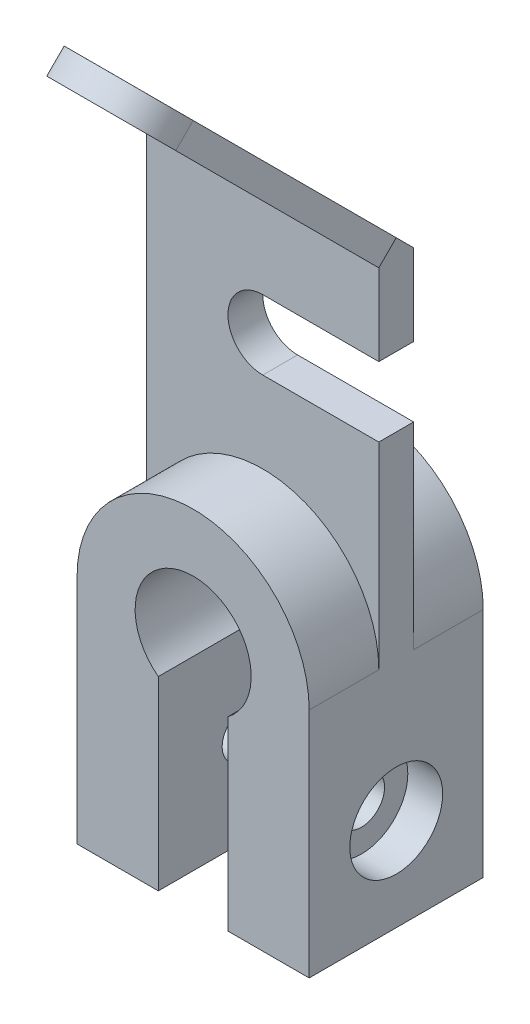
ISO-10303-21;
HEADER;
FILE_DESCRIPTION(('STEP AP214'),'2;1');
FILE_NAME('part.step','',(''),(''),'','','');
FILE_SCHEMA(('AUTOMOTIVE_DESIGN { 1 0 10303 214 1 1 1 1 }'));
ENDSEC;
DATA;
#1=APPLICATION_CONTEXT('core data for automotive mechanical design processes');
#2=APPLICATION_PROTOCOL_DEFINITION('international standard','automotive_design',2000,#1);
#3=PRODUCT_CONTEXT('',#1,'mechanical');
#4=PRODUCT('Part','Part','',(#3));
#5=PRODUCT_RELATED_PRODUCT_CATEGORY('part','',(#4));
#6=PRODUCT_DEFINITION_FORMATION('','',#4);
#7=PRODUCT_DEFINITION_CONTEXT('part definition',#1,'design');
#8=PRODUCT_DEFINITION('design','',#6,#7);
#9=PRODUCT_DEFINITION_SHAPE('','',#8);
#10=(LENGTH_UNIT() NAMED_UNIT(*) SI_UNIT(.MILLI.,.METRE.));
#11=(NAMED_UNIT(*) PLANE_ANGLE_UNIT() SI_UNIT($,.RADIAN.));
#12=(NAMED_UNIT(*) SI_UNIT($,.STERADIAN.) SOLID_ANGLE_UNIT());
#13=UNCERTAINTY_MEASURE_WITH_UNIT(LENGTH_MEASURE(1.E-05),#10,'distance_accuracy_value','');
#14=(GEOMETRIC_REPRESENTATION_CONTEXT(3) GLOBAL_UNCERTAINTY_ASSIGNED_CONTEXT((#13)) GLOBAL_UNIT_ASSIGNED_CONTEXT((#10,
#11,#12)) REPRESENTATION_CONTEXT('',''));
#15=CARTESIAN_POINT('',(0.,0.,0.));
#16=DIRECTION('',(0.,0.,1.));
#17=DIRECTION('',(1.,0.,0.));
#18=AXIS2_PLACEMENT_3D('',#15,#16,#17);
#19=CARTESIAN_POINT('',(30.,0.,22.5));
#20=DIRECTION('',(-1.,0.,0.));
#21=DIRECTION('',(0.,0.,1.));
#22=AXIS2_PLACEMENT_3D('',#19,#20,#21);
#23=PLANE('',#22);
#24=DIRECTION('',(0.,0.,1.));
#25=VECTOR('',#24,1.);
#26=CARTESIAN_POINT('',(30.,129.,-21.86));
#27=LINE('',#26,#25);
#28=CARTESIAN_POINT('',(30.,129.,-4.5));
#29=VERTEX_POINT('',#28);
#30=CARTESIAN_POINT('',(30.,129.,4.5));
#31=VERTEX_POINT('',#30);
#32=EDGE_CURVE('E188',#29,#31,#27,.T.);
#33=ORIENTED_EDGE('',*,*,#32,.F.);
#34=DIRECTION('',(0.,1.,0.));
#35=VECTOR('',#34,1.);
#36=CARTESIAN_POINT('',(30.,150.,-4.5));
#37=LINE('',#36,#35);
#38=CARTESIAN_POINT('',(30.,150.,-4.5));
#39=VERTEX_POINT('',#38);
#40=EDGE_CURVE('E257',#29,#39,#37,.T.);
#41=ORIENTED_EDGE('',*,*,#40,.T.);
#42=DIRECTION('',(0.,0.707106781186555,0.70710678118654));
#43=VECTOR('',#42,1.);
#44=CARTESIAN_POINT('',(30.,187.476659402887,32.9766594028869));
#45=LINE('',#44,#43);
#46=CARTESIAN_POINT('',(30.,154.499999999999,0.));
#47=VERTEX_POINT('',#46);
#48=EDGE_CURVE('E236',#39,#47,#45,.T.);
#49=ORIENTED_EDGE('',*,*,#48,.T.);
#50=DIRECTION('',(0.,-0.707106781186548,0.707106781186547));
#51=VECTOR('',#50,1.);
#52=CARTESIAN_POINT('',(30.,156.363961030678,-1.86396103067888));
#53=LINE('',#52,#51);
#54=CARTESIAN_POINT('',(30.,149.999999999999,4.50000000000005));
#55=VERTEX_POINT('',#54);
#56=EDGE_CURVE('E219',#47,#55,#53,.T.);
#57=ORIENTED_EDGE('',*,*,#56,.T.);
#58=DIRECTION('',(0.,1.,0.));
#59=VECTOR('',#58,1.);
#60=CARTESIAN_POINT('',(30.,150.,4.5));
#61=LINE('',#60,#59);
#62=EDGE_CURVE('E246',#31,#55,#61,.T.);
#63=ORIENTED_EDGE('',*,*,#62,.F.);
#64=EDGE_LOOP('',(#33,#41,#49,#57,#63));
#65=FACE_BOUND('',#64,.T.);
#66=ADVANCED_FACE('F39',(#65),#23,.F.);
#67=CARTESIAN_POINT('',(0.,60.,4.5));
#68=DIRECTION('',(0.,0.,1.));
#69=DIRECTION('',(1.,0.,0.));
#70=AXIS2_PLACEMENT_3D('',#67,#68,#69);
#71=PLANE('',#70);
#72=CARTESIAN_POINT('',(0.,120.,4.5));
#73=DIRECTION('',(0.,0.,1.));
#74=DIRECTION('',(1.,0.,0.));
#75=AXIS2_PLACEMENT_3D('',#72,#73,#74);
#76=CIRCLE('',#75,9.);
#77=CARTESIAN_POINT('',(0.,129.,4.5));
#78=VERTEX_POINT('',#77);
#79=CARTESIAN_POINT('',(0.,111.,4.5));
#80=VERTEX_POINT('',#79);
#81=EDGE_CURVE('E178',#78,#80,#76,.T.);
#82=ORIENTED_EDGE('',*,*,#81,.F.);
#83=DIRECTION('',(1.,0.,0.));
#84=VECTOR('',#83,1.);
#85=CARTESIAN_POINT('',(0.,129.,4.5));
#86=LINE('',#85,#84);
#87=EDGE_CURVE('E190',#78,#31,#86,.T.);
#88=ORIENTED_EDGE('',*,*,#87,.T.);
#89=ORIENTED_EDGE('',*,*,#62,.T.);
#90=DIRECTION('',(-1.,0.,0.));
#91=VECTOR('',#90,1.);
#92=CARTESIAN_POINT('',(-30.,150.,4.5));
#93=LINE('',#92,#91);
#94=CARTESIAN_POINT('',(-30.,149.999999999999,4.50000000000005));
#95=VERTEX_POINT('',#94);
#96=EDGE_CURVE('E249',#55,#95,#93,.T.);
#97=ORIENTED_EDGE('',*,*,#96,.T.);
#98=DIRECTION('',(0.,-1.,0.));
#99=VECTOR('',#98,1.);
#100=CARTESIAN_POINT('',(-30.,60.,4.5));
#101=LINE('',#100,#99);
#102=CARTESIAN_POINT('',(-30.,60.,4.5));
#103=VERTEX_POINT('',#102);
#104=EDGE_CURVE('E254',#95,#103,#101,.T.);
#105=ORIENTED_EDGE('',*,*,#104,.T.);
#106=CARTESIAN_POINT('',(0.,60.,4.5));
#107=DIRECTION('',(0.,0.,-1.));
#108=DIRECTION('',(1.,0.,0.));
#109=AXIS2_PLACEMENT_3D('',#106,#107,#108);
#110=CIRCLE('',#109,30.);
#111=CARTESIAN_POINT('',(30.,60.,4.5));
#112=VERTEX_POINT('',#111);
#113=EDGE_CURVE('E243',#103,#112,#110,.T.);
#114=ORIENTED_EDGE('',*,*,#113,.T.);
#115=CARTESIAN_POINT('',(30.,111.,4.5));
#116=VERTEX_POINT('',#115);
#117=EDGE_CURVE('E247',#112,#116,#61,.T.);
#118=ORIENTED_EDGE('',*,*,#117,.T.);
#119=DIRECTION('',(1.,0.,0.));
#120=VECTOR('',#119,1.);
#121=CARTESIAN_POINT('',(0.,111.,4.5));
#122=LINE('',#121,#120);
#123=EDGE_CURVE('E183',#80,#116,#122,.T.);
#124=ORIENTED_EDGE('',*,*,#123,.F.);
#125=EDGE_LOOP('',(#82,#88,#89,#97,#105,#114,#118,#124));
#126=FACE_BOUND('',#125,.T.);
#127=ADVANCED_FACE('F193',(#126),#71,.T.);
#128=CARTESIAN_POINT('',(0.,60.,-4.5));
#129=DIRECTION('',(0.,0.,1.));
#130=DIRECTION('',(1.,0.,0.));
#131=AXIS2_PLACEMENT_3D('',#128,#129,#130);
#132=PLANE('',#131);
#133=DIRECTION('',(1.,0.,0.));
#134=VECTOR('',#133,1.);
#135=CARTESIAN_POINT('',(0.,129.,-4.5));
#136=LINE('',#135,#134);
#137=CARTESIAN_POINT('',(0.,129.,-4.5));
#138=VERTEX_POINT('',#137);
#139=EDGE_CURVE('E11',#138,#29,#136,.T.);
#140=ORIENTED_EDGE('',*,*,#139,.F.);
#141=CARTESIAN_POINT('',(0.,120.,-4.5));
#142=DIRECTION('',(0.,0.,1.));
#143=DIRECTION('',(1.,0.,0.));
#144=AXIS2_PLACEMENT_3D('',#141,#142,#143);
#145=CIRCLE('',#144,9.);
#146=CARTESIAN_POINT('',(0.,111.,-4.5));
#147=VERTEX_POINT('',#146);
#148=EDGE_CURVE('E181',#138,#147,#145,.T.);
#149=ORIENTED_EDGE('',*,*,#148,.T.);
#150=DIRECTION('',(1.,0.,0.));
#151=VECTOR('',#150,1.);
#152=CARTESIAN_POINT('',(0.,111.,-4.5));
#153=LINE('',#152,#151);
#154=CARTESIAN_POINT('',(30.,111.,-4.5));
#155=VERTEX_POINT('',#154);
#156=EDGE_CURVE('E50',#147,#155,#153,.T.);
#157=ORIENTED_EDGE('',*,*,#156,.T.);
#158=CARTESIAN_POINT('',(30.,60.,-4.5));
#159=VERTEX_POINT('',#158);
#160=EDGE_CURVE('E258',#159,#155,#37,.T.);
#161=ORIENTED_EDGE('',*,*,#160,.F.);
#162=CARTESIAN_POINT('',(0.,60.,-4.5));
#163=DIRECTION('',(0.,0.,-1.));
#164=DIRECTION('',(1.,0.,0.));
#165=AXIS2_PLACEMENT_3D('',#162,#163,#164);
#166=CIRCLE('',#165,30.);
#167=CARTESIAN_POINT('',(-30.,60.,-4.49999999999999));
#168=VERTEX_POINT('',#167);
#169=EDGE_CURVE('E239',#168,#159,#166,.T.);
#170=ORIENTED_EDGE('',*,*,#169,.F.);
#171=DIRECTION('',(0.,-1.,0.));
#172=VECTOR('',#171,1.);
#173=CARTESIAN_POINT('',(-30.,60.,-4.5));
#174=LINE('',#173,#172);
#175=CARTESIAN_POINT('',(-30.,150.,-4.5));
#176=VERTEX_POINT('',#175);
#177=EDGE_CURVE('E250',#176,#168,#174,.T.);
#178=ORIENTED_EDGE('',*,*,#177,.F.);
#179=DIRECTION('',(-1.,0.,0.));
#180=VECTOR('',#179,1.);
#181=CARTESIAN_POINT('',(-30.,150.,-4.5));
#182=LINE('',#181,#180);
#183=EDGE_CURVE('E262',#39,#176,#182,.T.);
#184=ORIENTED_EDGE('',*,*,#183,.F.);
#185=ORIENTED_EDGE('',*,*,#40,.F.);
#186=EDGE_LOOP('',(#140,#149,#157,#161,#170,#178,#184,#185));
#187=FACE_BOUND('',#186,.T.);
#188=ADVANCED_FACE('F359',(#187),#132,.F.);
#189=CARTESIAN_POINT('',(0.,181.112698372208,48.3406204335662));
#190=DIRECTION('',(0.,0.707106781186548,-0.707106781186547));
#191=DIRECTION('',(0.,0.707106781186547,0.707106781186548));
#192=AXIS2_PLACEMENT_3D('',#189,#190,#191);
#193=CYLINDRICAL_SURFACE('',#192,15.);
#194=CARTESIAN_POINT('',(0.,191.973858531233,37.4794602745409));
#195=DIRECTION('',(0.,-0.707106781186548,0.707106781186547));
#196=DIRECTION('',(0.,-0.707106781186547,-0.707106781186548));
#197=AXIS2_PLACEMENT_3D('',#194,#195,#196);
#198=CIRCLE('',#197,15.);
#199=CARTESIAN_POINT('',(15.,191.973858531233,37.4794602745408));
#200=VERTEX_POINT('',#199);
#201=CARTESIAN_POINT('',(-15.,191.973858531233,37.4794602745408));
#202=VERTEX_POINT('',#201);
#203=EDGE_CURVE('E65',#200,#202,#198,.F.);
#204=ORIENTED_EDGE('',*,*,#203,.F.);
#205=DIRECTION('',(0.,-0.707106781186548,0.707106781186547));
#206=VECTOR('',#205,1.);
#207=CARTESIAN_POINT('',(15.,193.840620433566,35.6126983722083));
#208=LINE('',#207,#206);
#209=CARTESIAN_POINT('',(15.,191.976659402887,37.4766594028869));
#210=VERTEX_POINT('',#209);
#211=EDGE_CURVE('E230',#200,#210,#208,.F.);
#212=ORIENTED_EDGE('',*,*,#211,.T.);
#213=CARTESIAN_POINT('',(0.,191.976659402887,37.4766594028867));
#214=DIRECTION('',(0.,0.70710678118654,-0.707106781186555));
#215=DIRECTION('',(0.,0.707106781186555,0.70710678118654));
#216=AXIS2_PLACEMENT_3D('',#213,#214,#215);
#217=CIRCLE('',#216,15.);
#218=CARTESIAN_POINT('',(-15.,191.976659402887,37.4766594028867));
#219=VERTEX_POINT('',#218);
#220=EDGE_CURVE('E351',#210,#219,#217,.T.);
#221=ORIENTED_EDGE('',*,*,#220,.T.);
#222=DIRECTION('',(0.,-0.707106781186548,0.707106781186547));
#223=VECTOR('',#222,1.);
#224=CARTESIAN_POINT('',(-15.,193.840620433566,35.6126983722083));
#225=LINE('',#224,#223);
#226=EDGE_CURVE('E234',#219,#202,#225,.T.);
#227=ORIENTED_EDGE('',*,*,#226,.T.);
#228=EDGE_LOOP('',(#204,#212,#221,#227));
#229=FACE_BOUND('',#228,.T.);
#230=ADVANCED_FACE('F498',(#229),#193,.F.);
#231=CARTESIAN_POINT('',(0.,60.,22.5));
#232=DIRECTION('',(0.,0.,-1.));
#233=DIRECTION('',(-1.,0.,0.));
#234=AXIS2_PLACEMENT_3D('',#231,#232,#233);
#235=CYLINDRICAL_SURFACE('',#234,30.);
#236=ORIENTED_EDGE('',*,*,#169,.T.);
#237=DIRECTION('',(0.,0.,-1.));
#238=VECTOR('',#237,1.);
#239=CARTESIAN_POINT('',(30.,60.,22.5));
#240=LINE('',#239,#238);
#241=CARTESIAN_POINT('',(30.,60.,-22.5));
#242=VERTEX_POINT('',#241);
#243=EDGE_CURVE('E335',#159,#242,#240,.T.);
#244=ORIENTED_EDGE('',*,*,#243,.T.);
#245=CARTESIAN_POINT('',(0.,60.,-22.5));
#246=DIRECTION('',(0.,0.,1.));
#247=DIRECTION('',(1.,0.,0.));
#248=AXIS2_PLACEMENT_3D('',#245,#246,#247);
#249=CIRCLE('',#248,30.);
#250=CARTESIAN_POINT('',(-30.,60.,-22.5));
#251=VERTEX_POINT('',#250);
#252=EDGE_CURVE('E322',#242,#251,#249,.T.);
#253=ORIENTED_EDGE('',*,*,#252,.T.);
#254=DIRECTION('',(0.,0.,-1.));
#255=VECTOR('',#254,1.);
#256=CARTESIAN_POINT('',(-30.,60.,22.5));
#257=LINE('',#256,#255);
#258=EDGE_CURVE('E331',#168,#251,#257,.T.);
#259=ORIENTED_EDGE('',*,*,#258,.F.);
#260=EDGE_LOOP('',(#236,#244,#253,#259));
#261=FACE_BOUND('',#260,.T.);
#262=ADVANCED_FACE('F368',(#261),#235,.T.);
#263=CARTESIAN_POINT('',(0.,0.,22.5));
#264=DIRECTION('',(0.,1.,0.));
#265=DIRECTION('',(0.,0.,1.));
#266=AXIS2_PLACEMENT_3D('',#263,#264,#265);
#267=PLANE('',#266);
#268=DIRECTION('',(1.,0.,0.));
#269=VECTOR('',#268,1.);
#270=CARTESIAN_POINT('',(0.,0.,-22.5));
#271=LINE('',#270,#269);
#272=CARTESIAN_POINT('',(-30.,0.,-22.5));
#273=VERTEX_POINT('',#272);
#274=CARTESIAN_POINT('',(-9.,0.,-22.5));
#275=VERTEX_POINT('',#274);
#276=EDGE_CURVE('E320',#273,#275,#271,.T.);
#277=ORIENTED_EDGE('',*,*,#276,.T.);
#278=DIRECTION('',(0.,0.,1.));
#279=VECTOR('',#278,1.);
#280=CARTESIAN_POINT('',(-9.,0.,-41.5));
#281=LINE('',#280,#279);
#282=CARTESIAN_POINT('',(-9.,0.,22.5));
#283=VERTEX_POINT('',#282);
#284=EDGE_CURVE('E300',#275,#283,#281,.T.);
#285=ORIENTED_EDGE('',*,*,#284,.T.);
#286=DIRECTION('',(1.,0.,0.));
#287=VECTOR('',#286,1.);
#288=CARTESIAN_POINT('',(-30.,0.,22.5));
#289=LINE('',#288,#287);
#290=CARTESIAN_POINT('',(-30.,0.,22.5));
#291=VERTEX_POINT('',#290);
#292=EDGE_CURVE('E306',#291,#283,#289,.T.);
#293=ORIENTED_EDGE('',*,*,#292,.F.);
#294=DIRECTION('',(0.,0.,-1.));
#295=VECTOR('',#294,1.);
#296=CARTESIAN_POINT('',(-30.,0.,22.5));
#297=LINE('',#296,#295);
#298=EDGE_CURVE('E317',#291,#273,#297,.T.);
#299=ORIENTED_EDGE('',*,*,#298,.T.);
#300=EDGE_LOOP('',(#277,#285,#293,#299));
#301=FACE_BOUND('',#300,.T.);
#302=ADVANCED_FACE('F427',(#301),#267,.F.);
#303=CARTESIAN_POINT('',(9.,0.,22.5));
#304=VERTEX_POINT('',#303);
#305=CARTESIAN_POINT('',(30.,0.,22.5));
#306=VERTEX_POINT('',#305);
#307=EDGE_CURVE('E309',#304,#306,#289,.T.);
#308=ORIENTED_EDGE('',*,*,#307,.F.);
#309=DIRECTION('',(0.,0.,1.));
#310=VECTOR('',#309,1.);
#311=CARTESIAN_POINT('',(9.,0.,-41.5));
#312=LINE('',#311,#310);
#313=CARTESIAN_POINT('',(9.,0.,-22.5));
#314=VERTEX_POINT('',#313);
#315=EDGE_CURVE('E298',#314,#304,#312,.T.);
#316=ORIENTED_EDGE('',*,*,#315,.F.);
#317=CARTESIAN_POINT('',(30.,0.,-22.5));
#318=VERTEX_POINT('',#317);
#319=EDGE_CURVE('E297',#314,#318,#271,.T.);
#320=ORIENTED_EDGE('',*,*,#319,.T.);
#321=DIRECTION('',(0.,0.,-1.));
#322=VECTOR('',#321,1.);
#323=CARTESIAN_POINT('',(30.,0.,22.5));
#324=LINE('',#323,#322);
#325=EDGE_CURVE('E339',#306,#318,#324,.T.);
#326=ORIENTED_EDGE('',*,*,#325,.F.);
#327=EDGE_LOOP('',(#308,#316,#320,#326));
#328=FACE_BOUND('',#327,.T.);
#329=ADVANCED_FACE('F41',(#328),#267,.F.);
#330=CARTESIAN_POINT('',(30.,24.,0.));
#331=DIRECTION('',(1.,0.,0.));
#332=DIRECTION('',(0.,0.,-1.));
#333=AXIS2_PLACEMENT_3D('',#330,#331,#332);
#334=CIRCLE('',#333,12.);
#335=CARTESIAN_POINT('',(30.,24.,-12.));
#336=VERTEX_POINT('',#335);
#337=EDGE_CURVE('E276',#336,#336,#334,.T.);
#338=ORIENTED_EDGE('',*,*,#337,.F.);
#339=EDGE_LOOP('',(#338));
#340=FACE_BOUND('',#339,.T.);
#341=ORIENTED_EDGE('',*,*,#160,.T.);
#342=DIRECTION('',(0.,0.,1.));
#343=VECTOR('',#342,1.);
#344=CARTESIAN_POINT('',(30.,111.,-21.86));
#345=LINE('',#344,#343);
#346=EDGE_CURVE('E201',#155,#116,#345,.T.);
#347=ORIENTED_EDGE('',*,*,#346,.T.);
#348=ORIENTED_EDGE('',*,*,#117,.F.);
#349=CARTESIAN_POINT('',(30.,60.,22.5));
#350=VERTEX_POINT('',#349);
#351=EDGE_CURVE('E337',#350,#112,#240,.T.);
#352=ORIENTED_EDGE('',*,*,#351,.F.);
#353=DIRECTION('',(0.,1.,0.));
#354=VECTOR('',#353,1.);
#355=CARTESIAN_POINT('',(30.,0.,22.5));
#356=LINE('',#355,#354);
#357=EDGE_CURVE('E307',#306,#350,#356,.T.);
#358=ORIENTED_EDGE('',*,*,#357,.F.);
#359=ORIENTED_EDGE('',*,*,#325,.T.);
#360=DIRECTION('',(0.,1.,0.));
#361=VECTOR('',#360,1.);
#362=CARTESIAN_POINT('',(30.,0.,-22.5));
#363=LINE('',#362,#361);
#364=EDGE_CURVE('E318',#318,#242,#363,.T.);
#365=ORIENTED_EDGE('',*,*,#364,.T.);
#366=ORIENTED_EDGE('',*,*,#243,.F.);
#367=EDGE_LOOP('',(#341,#347,#348,#352,#358,#359,#365,#366));
#368=FACE_BOUND('',#367,.T.);
#369=ADVANCED_FACE('F364',(#340,#368),#23,.F.);
#370=ORIENTED_EDGE('',*,*,#351,.T.);
#371=ORIENTED_EDGE('',*,*,#113,.F.);
#372=CARTESIAN_POINT('',(-30.,60.,22.5));
#373=VERTEX_POINT('',#372);
#374=EDGE_CURVE('E332',#373,#103,#257,.T.);
#375=ORIENTED_EDGE('',*,*,#374,.F.);
#376=CARTESIAN_POINT('',(0.,60.,22.5));
#377=DIRECTION('',(0.,0.,1.));
#378=DIRECTION('',(1.,0.,0.));
#379=AXIS2_PLACEMENT_3D('',#376,#377,#378);
#380=CIRCLE('',#379,30.);
#381=EDGE_CURVE('E315',#350,#373,#380,.T.);
#382=ORIENTED_EDGE('',*,*,#381,.F.);
#383=EDGE_LOOP('',(#370,#371,#375,#382));
#384=FACE_BOUND('',#383,.T.);
#385=ADVANCED_FACE('F423',(#384),#235,.T.);
#386=CARTESIAN_POINT('',(-30.,60.,22.5));
#387=DIRECTION('',(1.,0.,0.));
#388=DIRECTION('',(0.,0.,-1.));
#389=AXIS2_PLACEMENT_3D('',#386,#387,#388);
#390=PLANE('',#389);
#391=CARTESIAN_POINT('',(-30.,24.,0.));
#392=DIRECTION('',(-1.,0.,0.));
#393=DIRECTION('',(0.,0.,1.));
#394=AXIS2_PLACEMENT_3D('',#391,#392,#393);
#395=CIRCLE('',#394,12.);
#396=CARTESIAN_POINT('',(-30.,24.,12.));
#397=VERTEX_POINT('',#396);
#398=EDGE_CURVE('E279',#397,#397,#395,.T.);
#399=ORIENTED_EDGE('',*,*,#398,.F.);
#400=EDGE_LOOP('',(#399));
#401=FACE_BOUND('',#400,.T.);
#402=ORIENTED_EDGE('',*,*,#104,.F.);
#403=DIRECTION('',(0.,-0.707106781186548,0.707106781186547));
#404=VECTOR('',#403,1.);
#405=CARTESIAN_POINT('',(-30.,156.363961030678,-1.86396103067888));
#406=LINE('',#405,#404);
#407=CARTESIAN_POINT('',(-30.,154.499999999999,0.));
#408=VERTEX_POINT('',#407);
#409=EDGE_CURVE('E217',#408,#95,#406,.T.);
#410=ORIENTED_EDGE('',*,*,#409,.F.);
#411=DIRECTION('',(0.,0.707106781186549,0.707106781186546));
#412=VECTOR('',#411,1.);
#413=CARTESIAN_POINT('',(-30.,150.,-4.5));
#414=LINE('',#413,#412);
#415=EDGE_CURVE('E240',#176,#408,#414,.T.);
#416=ORIENTED_EDGE('',*,*,#415,.F.);
#417=ORIENTED_EDGE('',*,*,#177,.T.);
#418=ORIENTED_EDGE('',*,*,#258,.T.);
#419=DIRECTION('',(0.,-1.,0.));
#420=VECTOR('',#419,1.);
#421=CARTESIAN_POINT('',(-30.,60.,-22.5));
#422=LINE('',#421,#420);
#423=EDGE_CURVE('E326',#251,#273,#422,.T.);
#424=ORIENTED_EDGE('',*,*,#423,.T.);
#425=ORIENTED_EDGE('',*,*,#298,.F.);
#426=DIRECTION('',(0.,-1.,0.));
#427=VECTOR('',#426,1.);
#428=CARTESIAN_POINT('',(-30.,60.,22.5));
#429=LINE('',#428,#427);
#430=EDGE_CURVE('E313',#373,#291,#429,.T.);
#431=ORIENTED_EDGE('',*,*,#430,.F.);
#432=ORIENTED_EDGE('',*,*,#374,.T.);
#433=EDGE_LOOP('',(#402,#410,#416,#417,#418,#424,#425,#431,#432));
#434=FACE_BOUND('',#433,.T.);
#435=ADVANCED_FACE('F374',(#401,#434),#390,.F.);
#436=CARTESIAN_POINT('',(0.,60.,22.5));
#437=DIRECTION('',(0.,0.,1.));
#438=DIRECTION('',(1.,0.,0.));
#439=AXIS2_PLACEMENT_3D('',#436,#437,#438);
#440=PLANE('',#439);
#441=DIRECTION('',(0.,-1.,0.));
#442=VECTOR('',#441,1.);
#443=CARTESIAN_POINT('',(-9.,48.,22.5));
#444=LINE('',#443,#442);
#445=CARTESIAN_POINT('',(-9.,48.,22.5));
#446=VERTEX_POINT('',#445);
#447=EDGE_CURVE('E295',#446,#283,#444,.T.);
#448=ORIENTED_EDGE('',*,*,#447,.F.);
#449=CARTESIAN_POINT('',(0.,60.,22.5));
#450=DIRECTION('',(0.,0.,1.));
#451=DIRECTION('',(1.,0.,0.));
#452=AXIS2_PLACEMENT_3D('',#449,#450,#451);
#453=CIRCLE('',#452,15.);
#454=CARTESIAN_POINT('',(9.,48.,22.5));
#455=VERTEX_POINT('',#454);
#456=EDGE_CURVE('E293',#455,#446,#453,.T.);
#457=ORIENTED_EDGE('',*,*,#456,.F.);
#458=DIRECTION('',(0.,1.,0.));
#459=VECTOR('',#458,1.);
#460=CARTESIAN_POINT('',(9.,0.,22.5));
#461=LINE('',#460,#459);
#462=EDGE_CURVE('E286',#304,#455,#461,.T.);
#463=ORIENTED_EDGE('',*,*,#462,.F.);
#464=ORIENTED_EDGE('',*,*,#307,.T.);
#465=ORIENTED_EDGE('',*,*,#357,.T.);
#466=ORIENTED_EDGE('',*,*,#381,.T.);
#467=ORIENTED_EDGE('',*,*,#430,.T.);
#468=ORIENTED_EDGE('',*,*,#292,.T.);
#469=EDGE_LOOP('',(#448,#457,#463,#464,#465,#466,#467,#468));
#470=FACE_BOUND('',#469,.T.);
#471=ADVANCED_FACE('F469',(#470),#440,.T.);
#472=CARTESIAN_POINT('',(0.,60.,-22.5));
#473=DIRECTION('',(0.,0.,1.));
#474=DIRECTION('',(1.,0.,0.));
#475=AXIS2_PLACEMENT_3D('',#472,#473,#474);
#476=PLANE('',#475);
#477=CARTESIAN_POINT('',(0.,60.,-22.5));
#478=DIRECTION('',(0.,0.,1.));
#479=DIRECTION('',(1.,0.,0.));
#480=AXIS2_PLACEMENT_3D('',#477,#478,#479);
#481=CIRCLE('',#480,15.);
#482=CARTESIAN_POINT('',(9.,48.,-22.5));
#483=VERTEX_POINT('',#482);
#484=CARTESIAN_POINT('',(-9.,48.,-22.5));
#485=VERTEX_POINT('',#484);
#486=EDGE_CURVE('E344',#483,#485,#481,.T.);
#487=ORIENTED_EDGE('',*,*,#486,.T.);
#488=DIRECTION('',(0.,-1.,0.));
#489=VECTOR('',#488,1.);
#490=CARTESIAN_POINT('',(-9.,60.,-22.5));
#491=LINE('',#490,#489);
#492=EDGE_CURVE('E349',#485,#275,#491,.T.);
#493=ORIENTED_EDGE('',*,*,#492,.T.);
#494=ORIENTED_EDGE('',*,*,#276,.F.);
#495=ORIENTED_EDGE('',*,*,#423,.F.);
#496=ORIENTED_EDGE('',*,*,#252,.F.);
#497=ORIENTED_EDGE('',*,*,#364,.F.);
#498=ORIENTED_EDGE('',*,*,#319,.F.);
#499=DIRECTION('',(0.,1.,0.));
#500=VECTOR('',#499,1.);
#501=CARTESIAN_POINT('',(9.,60.,-22.5));
#502=LINE('',#501,#500);
#503=EDGE_CURVE('E345',#314,#483,#502,.T.);
#504=ORIENTED_EDGE('',*,*,#503,.T.);
#505=EDGE_LOOP('',(#487,#493,#494,#495,#496,#497,#498,#504));
#506=FACE_BOUND('',#505,.T.);
#507=ADVANCED_FACE('F461',(#506),#476,.F.);
#508=CARTESIAN_POINT('',(-9.,48.,-41.5));
#509=DIRECTION('',(-1.,0.,0.));
#510=DIRECTION('',(0.,0.,1.));
#511=AXIS2_PLACEMENT_3D('',#508,#509,#510);
#512=PLANE('',#511);
#513=CARTESIAN_POINT('',(-9.,24.,0.));
#514=DIRECTION('',(-1.,0.,0.));
#515=DIRECTION('',(0.,0.,1.));
#516=AXIS2_PLACEMENT_3D('',#513,#514,#515);
#517=CIRCLE('',#516,6.);
#518=CARTESIAN_POINT('',(-9.,24.,6.));
#519=VERTEX_POINT('',#518);
#520=EDGE_CURVE('E271',#519,#519,#517,.T.);
#521=ORIENTED_EDGE('',*,*,#520,.T.);
#522=EDGE_LOOP('',(#521));
#523=FACE_BOUND('',#522,.T.);
#524=DIRECTION('',(0.,0.,1.));
#525=VECTOR('',#524,1.);
#526=CARTESIAN_POINT('',(-9.,48.,-41.5));
#527=LINE('',#526,#525);
#528=EDGE_CURVE('E301',#485,#446,#527,.T.);
#529=ORIENTED_EDGE('',*,*,#528,.T.);
#530=ORIENTED_EDGE('',*,*,#447,.T.);
#531=ORIENTED_EDGE('',*,*,#284,.F.);
#532=ORIENTED_EDGE('',*,*,#492,.F.);
#533=EDGE_LOOP('',(#529,#530,#531,#532));
#534=FACE_BOUND('',#533,.T.);
#535=ADVANCED_FACE('F459',(#523,#534),#512,.F.);
#536=CARTESIAN_POINT('',(0.,60.,-41.5));
#537=DIRECTION('',(0.,0.,1.));
#538=DIRECTION('',(1.,0.,0.));
#539=AXIS2_PLACEMENT_3D('',#536,#537,#538);
#540=CYLINDRICAL_SURFACE('',#539,15.);
#541=DIRECTION('',(0.,0.,1.));
#542=VECTOR('',#541,1.);
#543=CARTESIAN_POINT('',(9.,48.,-41.5));
#544=LINE('',#543,#542);
#545=EDGE_CURVE('E303',#483,#455,#544,.T.);
#546=ORIENTED_EDGE('',*,*,#545,.T.);
#547=ORIENTED_EDGE('',*,*,#456,.T.);
#548=ORIENTED_EDGE('',*,*,#528,.F.);
#549=ORIENTED_EDGE('',*,*,#486,.F.);
#550=EDGE_LOOP('',(#546,#547,#548,#549));
#551=FACE_BOUND('',#550,.T.);
#552=ADVANCED_FACE('F460',(#551),#540,.F.);
#553=CARTESIAN_POINT('',(9.,0.,-41.5));
#554=DIRECTION('',(1.,0.,0.));
#555=DIRECTION('',(0.,0.,-1.));
#556=AXIS2_PLACEMENT_3D('',#553,#554,#555);
#557=PLANE('',#556);
#558=CARTESIAN_POINT('',(9.,24.,0.));
#559=DIRECTION('',(1.,0.,0.));
#560=DIRECTION('',(0.,0.,-1.));
#561=AXIS2_PLACEMENT_3D('',#558,#559,#560);
#562=CIRCLE('',#561,6.);
#563=CARTESIAN_POINT('',(9.,24.,-6.));
#564=VERTEX_POINT('',#563);
#565=EDGE_CURVE('E270',#564,#564,#562,.T.);
#566=ORIENTED_EDGE('',*,*,#565,.T.);
#567=EDGE_LOOP('',(#566));
#568=FACE_BOUND('',#567,.T.);
#569=ORIENTED_EDGE('',*,*,#315,.T.);
#570=ORIENTED_EDGE('',*,*,#462,.T.);
#571=ORIENTED_EDGE('',*,*,#545,.F.);
#572=ORIENTED_EDGE('',*,*,#503,.F.);
#573=EDGE_LOOP('',(#569,#570,#571,#572));
#574=FACE_BOUND('',#573,.T.);
#575=ADVANCED_FACE('F456',(#568,#574),#557,.F.);
#576=CARTESIAN_POINT('',(-21.,24.,0.));
#577=DIRECTION('',(-1.,0.,0.));
#578=DIRECTION('',(0.,0.,1.));
#579=AXIS2_PLACEMENT_3D('',#576,#577,#578);
#580=CYLINDRICAL_SURFACE('',#579,12.);
#581=CARTESIAN_POINT('',(-21.,24.,0.));
#582=DIRECTION('',(-1.,0.,0.));
#583=DIRECTION('',(0.,0.,1.));
#584=AXIS2_PLACEMENT_3D('',#581,#582,#583);
#585=CIRCLE('',#584,12.);
#586=CARTESIAN_POINT('',(-21.,24.,12.));
#587=VERTEX_POINT('',#586);
#588=EDGE_CURVE('E284',#587,#587,#585,.T.);
#589=ORIENTED_EDGE('',*,*,#588,.F.);
#590=EDGE_LOOP('',(#589));
#591=FACE_BOUND('',#590,.T.);
#592=ORIENTED_EDGE('',*,*,#398,.T.);
#593=EDGE_LOOP('',(#592));
#594=FACE_BOUND('',#593,.T.);
#595=ADVANCED_FACE('F446',(#591,#594),#580,.F.);
#596=CARTESIAN_POINT('',(-21.,24.,0.));
#597=DIRECTION('',(-1.,0.,0.));
#598=DIRECTION('',(0.,0.,1.));
#599=AXIS2_PLACEMENT_3D('',#596,#597,#598);
#600=PLANE('',#599);
#601=CARTESIAN_POINT('',(-21.,24.,0.));
#602=DIRECTION('',(-1.,0.,0.));
#603=DIRECTION('',(0.,0.,1.));
#604=AXIS2_PLACEMENT_3D('',#601,#602,#603);
#605=CIRCLE('',#604,6.);
#606=CARTESIAN_POINT('',(-21.,24.,6.));
#607=VERTEX_POINT('',#606);
#608=EDGE_CURVE('E268',#607,#607,#605,.T.);
#609=ORIENTED_EDGE('',*,*,#608,.F.);
#610=EDGE_LOOP('',(#609));
#611=FACE_BOUND('',#610,.T.);
#612=ORIENTED_EDGE('',*,*,#588,.T.);
#613=EDGE_LOOP('',(#612));
#614=FACE_BOUND('',#613,.T.);
#615=ADVANCED_FACE('F440',(#611,#614),#600,.T.);
#616=CARTESIAN_POINT('',(21.,24.,0.));
#617=DIRECTION('',(1.,0.,0.));
#618=DIRECTION('',(0.,0.,-1.));
#619=AXIS2_PLACEMENT_3D('',#616,#617,#618);
#620=CYLINDRICAL_SURFACE('',#619,12.);
#621=CARTESIAN_POINT('',(21.,24.,0.));
#622=DIRECTION('',(1.,0.,0.));
#623=DIRECTION('',(0.,0.,-1.));
#624=AXIS2_PLACEMENT_3D('',#621,#622,#623);
#625=CIRCLE('',#624,12.);
#626=CARTESIAN_POINT('',(21.,24.,-12.));
#627=VERTEX_POINT('',#626);
#628=EDGE_CURVE('E280',#627,#627,#625,.T.);
#629=ORIENTED_EDGE('',*,*,#628,.F.);
#630=EDGE_LOOP('',(#629));
#631=FACE_BOUND('',#630,.T.);
#632=ORIENTED_EDGE('',*,*,#337,.T.);
#633=EDGE_LOOP('',(#632));
#634=FACE_BOUND('',#633,.T.);
#635=ADVANCED_FACE('F432',(#631,#634),#620,.F.);
#636=CARTESIAN_POINT('',(21.,24.,0.));
#637=DIRECTION('',(1.,0.,0.));
#638=DIRECTION('',(0.,0.,-1.));
#639=AXIS2_PLACEMENT_3D('',#636,#637,#638);
#640=PLANE('',#639);
#641=CARTESIAN_POINT('',(21.,24.,0.));
#642=DIRECTION('',(1.,0.,0.));
#643=DIRECTION('',(0.,0.,-1.));
#644=AXIS2_PLACEMENT_3D('',#641,#642,#643);
#645=CIRCLE('',#644,6.);
#646=CARTESIAN_POINT('',(21.,24.,-6.));
#647=VERTEX_POINT('',#646);
#648=EDGE_CURVE('E253',#647,#647,#645,.T.);
#649=ORIENTED_EDGE('',*,*,#648,.F.);
#650=EDGE_LOOP('',(#649));
#651=FACE_BOUND('',#650,.T.);
#652=ORIENTED_EDGE('',*,*,#628,.T.);
#653=EDGE_LOOP('',(#652));
#654=FACE_BOUND('',#653,.T.);
#655=ADVANCED_FACE('F436',(#651,#654),#640,.T.);
#656=CARTESIAN_POINT('',(-30.,24.,0.));
#657=DIRECTION('',(1.,0.,0.));
#658=DIRECTION('',(0.,0.,-1.));
#659=AXIS2_PLACEMENT_3D('',#656,#657,#658);
#660=CYLINDRICAL_SURFACE('',#659,6.);
#661=ORIENTED_EDGE('',*,*,#608,.T.);
#662=EDGE_LOOP('',(#661));
#663=FACE_BOUND('',#662,.T.);
#664=ORIENTED_EDGE('',*,*,#520,.F.);
#665=EDGE_LOOP('',(#664));
#666=FACE_BOUND('',#665,.T.);
#667=ADVANCED_FACE('F444',(#663,#666),#660,.F.);
#668=ORIENTED_EDGE('',*,*,#648,.T.);
#669=EDGE_LOOP('',(#668));
#670=FACE_BOUND('',#669,.T.);
#671=ORIENTED_EDGE('',*,*,#565,.F.);
#672=EDGE_LOOP('',(#671));
#673=FACE_BOUND('',#672,.T.);
#674=ADVANCED_FACE('F525',(#670,#673),#660,.F.);
#675=CARTESIAN_POINT('',(-30.,150.,4.5));
#676=DIRECTION('',(0.,-0.707106781186545,0.70710678118655));
#677=DIRECTION('',(0.,-0.70710678118655,-0.707106781186545));
#678=AXIS2_PLACEMENT_3D('',#675,#676,#677);
#679=PLANE('',#678);
#680=CARTESIAN_POINT('',(0.,187.476659402886,41.9766594028871));
#681=DIRECTION('',(0.,-0.707106781186548,0.707106781186547));
#682=DIRECTION('',(0.,-0.707106781186547,-0.707106781186548));
#683=AXIS2_PLACEMENT_3D('',#680,#681,#682);
#684=CIRCLE('',#683,7.50000000000001);
#685=CARTESIAN_POINT('',(0.,182.173358543987,36.673358543988));
#686=VERTEX_POINT('',#685);
#687=EDGE_CURVE('E200',#686,#686,#684,.T.);
#688=ORIENTED_EDGE('',*,*,#687,.F.);
#689=EDGE_LOOP('',(#688));
#690=FACE_BOUND('',#689,.T.);
#691=DIRECTION('',(0.272322465799349,-0.680382419901103,-0.680382419901104));
#692=VECTOR('',#691,1.);
#693=CARTESIAN_POINT('',(15.,187.476659402886,41.9766594028871));
#694=LINE('',#693,#692);
#695=CARTESIAN_POINT('',(15.,187.476659402886,41.9766594028871));
#696=VERTEX_POINT('',#695);
#697=EDGE_CURVE('E211',#696,#55,#694,.T.);
#698=ORIENTED_EDGE('',*,*,#697,.F.);
#699=CARTESIAN_POINT('',(0.,187.476659402886,41.9766594028871));
#700=DIRECTION('',(0.,-0.707106781186548,0.707106781186547));
#701=DIRECTION('',(0.,-0.707106781186547,-0.707106781186548));
#702=AXIS2_PLACEMENT_3D('',#699,#700,#701);
#703=CIRCLE('',#702,15.);
#704=CARTESIAN_POINT('',(-15.,187.476659402887,41.9766594028871));
#705=VERTEX_POINT('',#704);
#706=EDGE_CURVE('E215',#696,#705,#703,.T.);
#707=ORIENTED_EDGE('',*,*,#706,.T.);
#708=DIRECTION('',(0.272322465799349,0.680382419901103,0.680382419901104));
#709=VECTOR('',#708,1.);
#710=CARTESIAN_POINT('',(-15.,187.476659402886,41.9766594028871));
#711=LINE('',#710,#709);
#712=EDGE_CURVE('E214',#95,#705,#711,.T.);
#713=ORIENTED_EDGE('',*,*,#712,.F.);
#714=ORIENTED_EDGE('',*,*,#96,.F.);
#715=EDGE_LOOP('',(#698,#707,#713,#714));
#716=FACE_BOUND('',#715,.T.);
#717=ADVANCED_FACE('F391',(#690,#716),#679,.T.);
#718=CARTESIAN_POINT('',(-30.,187.476659402887,32.9766594028869));
#719=DIRECTION('',(0.,0.70710678118654,-0.707106781186555));
#720=DIRECTION('',(0.,0.707106781186555,0.70710678118654));
#721=AXIS2_PLACEMENT_3D('',#718,#719,#720);
#722=PLANE('',#721);
#723=DIRECTION('',(-0.272322465799349,-0.68038241990111,-0.680382419901096));
#724=VECTOR('',#723,1.);
#725=CARTESIAN_POINT('',(-17.7799436451515,185.031125992983,30.5311259929827));
#726=LINE('',#725,#724);
#727=EDGE_CURVE('E227',#219,#408,#726,.T.);
#728=ORIENTED_EDGE('',*,*,#727,.F.);
#729=ORIENTED_EDGE('',*,*,#220,.F.);
#730=DIRECTION('',(-0.272322465799349,0.68038241990111,0.680382419901096));
#731=VECTOR('',#730,1.);
#732=CARTESIAN_POINT('',(13.3303721224092,196.148131089423,41.6481310894223));
#733=LINE('',#732,#731);
#734=EDGE_CURVE('E220',#47,#210,#733,.T.);
#735=ORIENTED_EDGE('',*,*,#734,.F.);
#736=ORIENTED_EDGE('',*,*,#48,.F.);
#737=ORIENTED_EDGE('',*,*,#183,.T.);
#738=ORIENTED_EDGE('',*,*,#415,.T.);
#739=EDGE_LOOP('',(#728,#729,#735,#736,#737,#738));
#740=FACE_BOUND('',#739,.T.);
#741=ADVANCED_FACE('F378',(#740),#722,.T.);
#742=CARTESIAN_POINT('',(15.,193.840620433565,35.6126983722081));
#743=DIRECTION('',(-0.962206045824366,-0.192561062236161,-0.192561062236161));
#744=DIRECTION('',(-0.196233574983259,0.,0.980557180407797));
#745=AXIS2_PLACEMENT_3D('',#742,#743,#744);
#746=PLANE('',#745);
#747=ORIENTED_EDGE('',*,*,#734,.T.);
#748=ORIENTED_EDGE('',*,*,#211,.F.);
#749=EDGE_CURVE('E229',#696,#200,#208,.F.);
#750=ORIENTED_EDGE('',*,*,#749,.F.);
#751=ORIENTED_EDGE('',*,*,#697,.T.);
#752=ORIENTED_EDGE('',*,*,#56,.F.);
#753=EDGE_LOOP('',(#747,#748,#750,#751,#752));
#754=FACE_BOUND('',#753,.T.);
#755=ADVANCED_FACE('F387',(#754),#746,.F.);
#756=CARTESIAN_POINT('',(-15.,193.840620433565,35.6126983722081));
#757=DIRECTION('',(0.962206045824366,-0.192561062236161,-0.192561062236161));
#758=DIRECTION('',(-0.196233574983259,0.,-0.980557180407797));
#759=AXIS2_PLACEMENT_3D('',#756,#757,#758);
#760=PLANE('',#759);
#761=ORIENTED_EDGE('',*,*,#727,.T.);
#762=ORIENTED_EDGE('',*,*,#409,.T.);
#763=ORIENTED_EDGE('',*,*,#712,.T.);
#764=EDGE_CURVE('E231',#202,#705,#225,.T.);
#765=ORIENTED_EDGE('',*,*,#764,.F.);
#766=ORIENTED_EDGE('',*,*,#226,.F.);
#767=EDGE_LOOP('',(#761,#762,#763,#765,#766));
#768=FACE_BOUND('',#767,.T.);
#769=ADVANCED_FACE('F395',(#768),#760,.F.);
#770=CARTESIAN_POINT('',(0.,191.973858531233,37.4794602745407));
#771=DIRECTION('',(0.,-0.707106781186548,0.707106781186547));
#772=DIRECTION('',(0.,-0.707106781186547,-0.707106781186548));
#773=AXIS2_PLACEMENT_3D('',#770,#771,#772);
#774=CYLINDRICAL_SURFACE('',#773,15.);
#775=ORIENTED_EDGE('',*,*,#749,.T.);
#776=CARTESIAN_POINT('',(0.,191.973858531233,37.4794602745407));
#777=DIRECTION('',(0.,-0.707106781186548,0.707106781186547));
#778=DIRECTION('',(0.,-0.707106781186547,-0.707106781186548));
#779=AXIS2_PLACEMENT_3D('',#776,#777,#778);
#780=CIRCLE('',#779,15.);
#781=EDGE_CURVE('E206',#200,#202,#780,.T.);
#782=ORIENTED_EDGE('',*,*,#781,.T.);
#783=ORIENTED_EDGE('',*,*,#764,.T.);
#784=ORIENTED_EDGE('',*,*,#706,.F.);
#785=EDGE_LOOP('',(#775,#782,#783,#784));
#786=FACE_BOUND('',#785,.T.);
#787=ADVANCED_FACE('F399',(#786),#774,.T.);
#788=CARTESIAN_POINT('',(0.,191.973858531233,37.4794602745407));
#789=DIRECTION('',(0.,-0.707106781186548,0.707106781186547));
#790=DIRECTION('',(0.,-0.707106781186547,-0.707106781186548));
#791=AXIS2_PLACEMENT_3D('',#788,#789,#790);
#792=PLANE('',#791);
#793=CARTESIAN_POINT('',(0.,191.973858531233,37.4794602745407));
#794=DIRECTION('',(0.,-0.707106781186548,0.707106781186547));
#795=DIRECTION('',(0.,-0.707106781186547,-0.707106781186548));
#796=AXIS2_PLACEMENT_3D('',#793,#794,#795);
#797=CIRCLE('',#796,7.50000000000001);
#798=CARTESIAN_POINT('',(0.,186.670557672334,32.1761594156415));
#799=VERTEX_POINT('',#798);
#800=EDGE_CURVE('E210',#799,#799,#797,.T.);
#801=ORIENTED_EDGE('',*,*,#800,.T.);
#802=EDGE_LOOP('',(#801));
#803=FACE_BOUND('',#802,.T.);
#804=ORIENTED_EDGE('',*,*,#781,.F.);
#805=ORIENTED_EDGE('',*,*,#203,.T.);
#806=EDGE_LOOP('',(#804,#805));
#807=FACE_BOUND('',#806,.T.);
#808=ADVANCED_FACE('F402',(#803,#807),#792,.F.);
#809=CARTESIAN_POINT('',(0.,206.115994154964,23.3373246508097));
#810=DIRECTION('',(0.,-0.707106781186548,0.707106781186547));
#811=DIRECTION('',(0.,-0.707106781186547,-0.707106781186548));
#812=AXIS2_PLACEMENT_3D('',#809,#810,#811);
#813=CYLINDRICAL_SURFACE('',#812,7.50000000000001);
#814=ORIENTED_EDGE('',*,*,#687,.T.);
#815=EDGE_LOOP('',(#814));
#816=FACE_BOUND('',#815,.T.);
#817=ORIENTED_EDGE('',*,*,#800,.F.);
#818=EDGE_LOOP('',(#817));
#819=FACE_BOUND('',#818,.T.);
#820=ADVANCED_FACE('F401',(#816,#819),#813,.F.);
#821=CARTESIAN_POINT('',(0.,129.,-21.86));
#822=DIRECTION('',(0.,-1.,0.));
#823=DIRECTION('',(0.,0.,-1.));
#824=AXIS2_PLACEMENT_3D('',#821,#822,#823);
#825=PLANE('',#824);
#826=ORIENTED_EDGE('',*,*,#139,.T.);
#827=ORIENTED_EDGE('',*,*,#32,.T.);
#828=ORIENTED_EDGE('',*,*,#87,.F.);
#829=DIRECTION('',(0.,0.,1.));
#830=VECTOR('',#829,1.);
#831=CARTESIAN_POINT('',(0.,129.,-21.86));
#832=LINE('',#831,#830);
#833=EDGE_CURVE('E172',#138,#78,#832,.T.);
#834=ORIENTED_EDGE('',*,*,#833,.F.);
#835=EDGE_LOOP('',(#826,#827,#828,#834));
#836=FACE_BOUND('',#835,.T.);
#837=ADVANCED_FACE('F189',(#836),#825,.T.);
#838=CARTESIAN_POINT('',(0.,111.,-21.86));
#839=DIRECTION('',(0.,-1.,0.));
#840=DIRECTION('',(0.,0.,-1.));
#841=AXIS2_PLACEMENT_3D('',#838,#839,#840);
#842=PLANE('',#841);
#843=DIRECTION('',(0.,0.,1.));
#844=VECTOR('',#843,1.);
#845=CARTESIAN_POINT('',(0.,111.,-21.86));
#846=LINE('',#845,#844);
#847=EDGE_CURVE('E53',#147,#80,#846,.T.);
#848=ORIENTED_EDGE('',*,*,#847,.T.);
#849=ORIENTED_EDGE('',*,*,#123,.T.);
#850=ORIENTED_EDGE('',*,*,#346,.F.);
#851=ORIENTED_EDGE('',*,*,#156,.F.);
#852=EDGE_LOOP('',(#848,#849,#850,#851));
#853=FACE_BOUND('',#852,.T.);
#854=ADVANCED_FACE('F701',(#853),#842,.F.);
#855=CARTESIAN_POINT('',(0.,120.,-21.86));
#856=DIRECTION('',(0.,0.,1.));
#857=DIRECTION('',(1.,0.,0.));
#858=AXIS2_PLACEMENT_3D('',#855,#856,#857);
#859=CYLINDRICAL_SURFACE('',#858,9.);
#860=ORIENTED_EDGE('',*,*,#833,.T.);
#861=ORIENTED_EDGE('',*,*,#81,.T.);
#862=ORIENTED_EDGE('',*,*,#847,.F.);
#863=ORIENTED_EDGE('',*,*,#148,.F.);
#864=EDGE_LOOP('',(#860,#861,#862,#863));
#865=FACE_BOUND('',#864,.T.);
#866=ADVANCED_FACE('F176',(#865),#859,.F.);
#867=CLOSED_SHELL('',(#66,#127,#188,#230,#262,#302,#329,#369,#385,#435,#471,#507,#535,#552,#575,
#595,#615,#635,#655,#667,#674,#717,#741,#755,#769,#787,#808,#820,#837,#854,#866));
#868=MANIFOLD_SOLID_BREP('B2',#867);
#869=ADVANCED_BREP_SHAPE_REPRESENTATION('',(#18,#868),#14);
#870=SHAPE_DEFINITION_REPRESENTATION(#9,#869);
ENDSEC;
END-ISO-10303-21;
